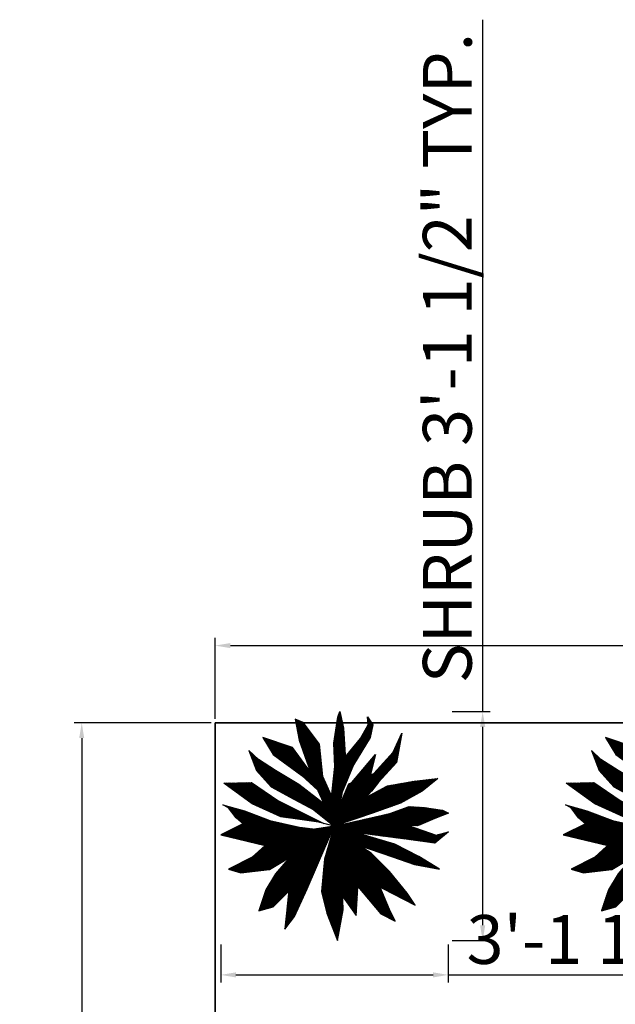
# Model space of a CAD drawing. Units: inches. Extents: x 1986 to 21484, y -1816 to 2016.
# Tile 48 of 85: x 3507 to 3604, y 1855 to 2016. Entities that reach past the tile are written whole.
import ezdxf

# ---------------------------------------------------------------- set-up
doc = ezdxf.new("R2010")
doc.units = ezdxf.units.IN
for name, color, linetype, lineweight in [('A-ANNO-DIMS', 2, 'Continuous', 18), ('C-PROP', 7, 'Continuous', 35), ('L-PLNT', 84, 'Continuous', 13), ('vfolhas', 114, 'Continuous', 5)]:
    doc.layers.add(name, color=color, linetype=linetype, lineweight=lineweight)
for name, color, linetype in [('vfolha', 72, 'Continuous'), ('vfolha2', 110, 'Continuous'), ('vfolhas2', 102, 'Continuous')]:
    doc.layers.add(name, color=color, linetype=linetype)
doc.styles.get("Standard").update_dxf_attribs({"font": 'arial.ttf'})
doc.dimstyles.new('ISO-25', dxfattribs={"dimtxt": 8, "dimasz": 2.5, "dimexe": 1.25, "dimexo": 0.625, "dimtad": 1, "dimdec": 1, "dimlunit": 3, "dimtxsty": 'Standard', "dimcen": 2.5, "dimadec": 0, "dimazin": 0, "dimtfac": 1, "dimtdec": 1, "dimtmove": 0, "dimatfit": 3, "dimfxl": 1, "dimarcsym": 0})
pattern_1 = [(45, (-2446.5133113, 50.986076), (-0.004419417382, 0.004419417382), [])]

# ---------------------------------------------------------------- blocks, each defined once
blk = doc.blocks.new('*D33')
at = {"layer": 'A-ANNO-DIMS', "color": 0, "lineweight": -2, "transparency": 16777216}
for p, q in [((3538.91, 1901.38), (3538.91, 1914.65)), ((3898.91, 1901.38), (3898.91, 1914.65)), ((3541.41, 1913.4), (3896.41, 1913.4))]:
    blk.add_line(p, q, dxfattribs=at)
at = {"layer": 'A-ANNO-DIMS', "color": 0, "transparency": 16777216}
for points in [[(3541.41, 1913.82), (3541.41, 1912.99), (3538.91, 1913.4)], [(3896.41, 1913.82), (3896.41, 1912.99), (3898.91, 1913.4)]]:
    blk.add_solid(points, dxfattribs=at)
at = {"layer": 'Defpoints', "color": 0, "transparency": 16777216}
for p in [(3898.91, 1913.4), (3538.91, 1900.75), (3898.91, 1900.75)]:
    blk.add_point(p, dxfattribs=at)
at = {"layer": 'A-ANNO-DIMS', "color": 0, "transparency": 16777216, "insert": (3718.91, 1918.12), "char_height": 8, "attachment_point": 5}
blk.add_mtext("30'", dxfattribs=at)
blk = doc.blocks.new('*D32')
at = {"layer": 'A-ANNO-DIMS', "color": 0, "lineweight": -2, "transparency": 16777216}
for p, q in [((3538.28, 1900.75), (3515.81, 1900.75)), ((3517.06, 1898.25), (3517.06, 1069.25)), ((3538.28, 1066.75), (3515.81, 1066.75))]:
    blk.add_line(p, q, dxfattribs=at)
at = {"layer": 'A-ANNO-DIMS', "color": 0, "transparency": 16777216}
for points in [[(3516.64, 1898.25), (3517.47, 1898.25), (3517.06, 1900.75)], [(3516.64, 1069.25), (3517.47, 1069.25), (3517.06, 1066.75)]]:
    blk.add_solid(points, dxfattribs=at)
at = {"layer": 'Defpoints', "color": 0, "transparency": 16777216}
for p in [(3538.91, 1900.75), (3517.06, 1066.75), (3538.91, 1066.75)]:
    blk.add_point(p, dxfattribs=at)
at = {"layer": 'A-ANNO-DIMS', "color": 0, "transparency": 16777216, "insert": (3512.35, 1483.75), "char_height": 8, "attachment_point": 5, "rotation": 90}
blk.add_mtext('69\'-6"', dxfattribs=at)
blk = doc.blocks.new('arbusto_PB_verde_grande')
at = {"layer": 'vfolha2'}
h = blk.add_hatch(dxfattribs=at)
h.set_pattern_fill('ANSI31', color=256, scale=0.05, style=0)
h.set_pattern_definition(pattern_1)
h.paths.add_polyline_path([(0.0294, 0.3565), (0.0003, 0.0905), (0.0263, -0.0393), (0.047, 0.0623), (0.0619, 0.0973), (0.0937, 0.2657), (0.0996, 0.4347), (0.0879, 0.6131), (0.0645, 0.7227), (0.0499, 0.6851), (0.0236, 0.5129)])
h.paths.add_polyline_path([(0.3011, 0.4379), (0.1423, 0.2487), (0.2669, 0.3002)])
h.paths.add_polyline_path([(0.38, 0.2282), (0.237, 0.1519), (0.1843, 0.0936), (0.1112, 0.0436), (0.0263, -0.0393), (0.2806, 0.0467), (0.3683, 0.078), (0.4676, 0.1124), (0.6107, 0.1938), (0.7159, 0.2782), (0.5581, 0.2595)])
h.paths.add_polyline_path([(0.561, -0.2944), (0.7275, -0.3257), (0.5902, -0.2412), (0.4296, -0.1598), (0.0263, -0.0393), (0.1492, -0.1411), (0.1884, -0.166), (0.415, -0.2444)])
h.paths.add_polyline_path([(-0.2743, -0.4478), (-0.3035, -0.7263), (-0.2392, -0.6417), (-0.1546, -0.4572), (0.0263, -0.0393), (-0.1633, -0.2538)])
h.paths.add_polyline_path([(-0.5196, -0.2474), (-0.6774, -0.3257), (-0.5956, -0.3507), (-0.4057, -0.3288), (-0.2101, -0.21), (0.0263, -0.0393), (-0.1487, -0.0659), (-0.3152, -0.091), (-0.4145, -0.1505)])
h.paths.add_polyline_path([(-0.5255, 0.2501), (-0.7095, 0.247), (-0.5196, 0.1093), (-0.3298, 0.0217), (-0.0757, -0.0128), (-0.0423, -0.0215), (-0.3502, 0.1312)])
h = blk.add_hatch(dxfattribs=at)
h.set_pattern_fill('ANSI31', color=256, scale=0.05, style=0)
h.set_pattern_definition(pattern_1)
h.paths.add_polyline_path([(-0.1896, 0.297), (-0.0855, 0.2019), (-0.1078, 0.2501), (-0.132, 0.3187), (-0.251, 0.4848), (-0.4495, 0.5505), (-0.3795, 0.4379)])
h.paths.add_polyline_path([(0.0791, -0.4071), (0.0821, -0.5063), (0.1726, -0.6355), (0.1843, -0.4415), (0.149, -0.2918), (0.0263, -0.0393), (0.0353, -0.2538)])
at = {"layer": 'vfolhas'}
h = blk.add_hatch(dxfattribs=at)
h.set_pattern_fill('ANSI31', color=256, scale=0.05, style=0)
h.set_pattern_definition(pattern_1)
h.paths.add_polyline_path([(-0.0728, 0.5067), (-0.1808, 0.6506), (-0.2334, 0.6725), (-0.2071, 0.5318), (-0.1078, 0.2501), (0.0263, -0.0393), (0.0003, 0.0905), (0.0082, 0.1624), (-0.0494, 0.2908)])
h.paths.add_polyline_path([(0.099, 0.4193), (0.0937, 0.2657), (0.0791, 0.1881), (0.1551, 0.369), (0.2661, 0.5505), (0.2836, 0.635), (0.2485, 0.6882), (0.2514, 0.635), (0.2018, 0.5443)])
h.paths.add_polyline_path([(0.1229, 0.2407), (0.047, 0.0623), (0.0263, -0.0393), (0.1112, 0.0436), (0.1843, 0.0936), (0.2748, 0.1938), (0.3215, 0.2532), (0.4413, 0.3847), (0.4763, 0.5787), (0.4179, 0.4535), (0.2894, 0.3095)])
h.paths.add_polyline_path([(0.5815, -0.0378), (0.7071, 0.0154), (0.7859, 0.0467), (0.748, 0.0655), (0.6282, 0.0842), (0.526, 0.0905), (0.3974, 0.0436), (0.0263, -0.0393), (0.2573, -0.0315), (0.4383, -0.0347)])
h.paths.add_polyline_path([(0.5202, -0.0365), (0.4383, -0.0347), (0.2573, -0.0315), (0.0263, -0.0393), (0.1796, -0.0852), (0.5377, -0.1317), (0.6954, -0.1536), (0.7859, -0.0785), (0.7041, -0.1004)])
h.paths.add_polyline_path([(0.2719, -0.2193), (0.1492, -0.1411), (0.0263, -0.0393), (0.1579, -0.3101), (0.2952, -0.4258), (0.4179, -0.4916), (0.564, -0.5667), (0.5114, -0.4853), (0.3946, -0.3414)])
h.paths.add_polyline_path([(-0.0582, -0.4759), (-0.0231, -0.6198), (0.047, -0.8013), (0.0849, -0.5979), (0.0791, -0.4071), (0.0353, -0.2538), (0.0263, -0.0393), (-0.0377, -0.26)])
h.paths.add_polyline_path([(-0.2422, 0.1405), (-0.1107, 0.0686), (0.0263, -0.0393), (-0.0423, 0.1087), (-0.2101, 0.2376), (-0.3649, 0.3314), (-0.4787, 0.4034), (-0.543, 0.4629), (-0.4904, 0.3314), (-0.3941, 0.2219)])
h = blk.add_hatch(dxfattribs=at)
h.set_pattern_fill('ANSI31', color=256, scale=0.05, style=0)
h.set_pattern_definition(pattern_1)
h.paths.add_polyline_path([(-0.5722, 0.0623), (-0.7153, 0.103), (-0.6774, 0.0811), (-0.6277, 0.0154), (-0.5635, -0.041), (-0.2646, -0.0834), (-0.1487, -0.0659), (-0.1015, -0.0588), (-0.2042, -0.0472), (-0.4028, -0.0034)])
h.paths.add_polyline_path([(-0.5635, -0.041), (-0.5828, -0.024), (-0.7299, -0.0973), (-0.4334, -0.1679), (-0.4145, -0.1505), (-0.3152, -0.091), (-0.2646, -0.0834)])
h.paths.add_polyline_path([(-0.2769, -0.4727), (-0.2743, -0.4478), (-0.1633, -0.2538), (0.0263, -0.0393), (-0.2101, -0.21), (-0.2672, -0.2447), (-0.3649, -0.357), (-0.4291, -0.4634), (-0.4759, -0.6043), (-0.3795, -0.576)])
h = blk.add_hatch(dxfattribs=at)
h.set_pattern_fill('ANSI31', color=256, scale=0.05, style=0)
h.set_pattern_definition(pattern_1)
h.paths.add_polyline_path([(0.3361, -0.623), (0.4325, -0.6731), (0.3946, -0.5948), (0.3303, -0.4446), (0.2952, -0.4258), (0.1579, -0.3101), (0.149, -0.2918), (0.1843, -0.4415)])
at = {"layer": 'vfolha'}
for p, q in [((0.0263, -0.0393), (-0.1487, -0.0659)), ((0.0263, -0.0393), (-0.0377, -0.26)), ((0.0353, -0.2538), (0.0263, -0.0393)), ((0.5202, -0.0365), (0.7041, -0.1004)), ((0.5377, -0.1317), (0.1796, -0.0852)), ((0.7859, -0.0785), (0.6954, -0.1536)), ((0.7041, -0.1004), (0.7859, -0.0785)), ((0.6954, -0.1536), (0.5377, -0.1317)), ((-0.2672, -0.2447), (-0.3649, -0.357)), ((-0.0377, -0.26), (-0.0582, -0.4759)), ((0.0791, -0.4071), (0.0353, -0.2538)), ((0.3946, -0.3414), (0.2719, -0.2193)), ((0.1579, -0.3101), (0.2952, -0.4258)), ((0.5114, -0.4853), (0.3946, -0.3414)), ((0.0849, -0.5979), (0.0791, -0.4071)), ((0.2952, -0.4258), (0.4179, -0.4916)), ((0.4179, -0.4916), (0.564, -0.5667)), ((0.564, -0.5667), (0.5114, -0.4853)), ((-0.0231, -0.6198), (0.047, -0.8013)), ((0.047, -0.8013), (0.0849, -0.5979))]:
    blk.add_line(p, q, dxfattribs=at)
at = {"layer": 'vfolha2'}
for p, q in [((0.0499, 0.6851), (0.0645, 0.7227)), ((0.0645, 0.7227), (0.0879, 0.6131)), ((0.0236, 0.5129), (0.0499, 0.6851)), ((0.0879, 0.6131), (0.0996, 0.4347)), ((-0.4495, 0.5505), (-0.3795, 0.4379)), ((-0.251, 0.4848), (-0.4495, 0.5505)), ((-0.132, 0.3187), (-0.251, 0.4848)), ((0.0294, 0.3565), (0.0236, 0.5129)), ((-0.3795, 0.4379), (-0.1896, 0.297)), ((0.0996, 0.4347), (0.0937, 0.2657)), ((0.1434, 0.2501), (0.3011, 0.4379)), ((0.3011, 0.4379), (0.2661, 0.297)), ((0.0003, 0.0905), (0.0294, 0.3565)), ((-0.1896, 0.297), (-0.0822, 0.1989)), ((0.5581, 0.2595), (0.7159, 0.2782)), ((0.7159, 0.2782), (0.6107, 0.1938)), ((-0.7095, 0.247), (-0.5255, 0.2501)), ((-0.5196, 0.1093), (-0.7095, 0.247)), ((-0.5255, 0.2501), (-0.3502, 0.1312)), ((0.237, 0.1519), (0.38, 0.2282)), ((0.38, 0.2282), (0.5581, 0.2595)), ((-0.3502, 0.1312), (-0.0423, -0.0215)), ((0.6107, 0.1938), (0.4676, 0.1124)), ((-0.3298, 0.0217), (-0.5196, 0.1093)), ((0.0263, -0.0393), (0.0003, 0.0905)), ((0.3683, 0.078), (0.2806, 0.0467)), ((-0.0757, -0.0128), (-0.3298, 0.0217)), ((0.2806, 0.0467), (0.0263, -0.0393)), ((-0.2101, -0.21), (0.0263, -0.0393)), ((0.0263, -0.0393), (-0.1633, -0.2538)), ((-0.1546, -0.4572), (0.0263, -0.0393)), ((0.4296, -0.1598), (0.0263, -0.0393)), ((0.0263, -0.0393), (0.1579, -0.3101)), ((-0.3152, -0.091), (-0.4145, -0.1505)), ((-0.1487, -0.0659), (-0.3152, -0.091)), ((-0.4145, -0.1505), (-0.5196, -0.2474)), ((0.1884, -0.166), (0.415, -0.2444)), ((0.5902, -0.2412), (0.4296, -0.1598)), ((-0.5196, -0.2474), (-0.6774, -0.3257)), ((-0.4057, -0.3288), (-0.2101, -0.21)), ((-0.1633, -0.2538), (-0.2743, -0.4478)), ((0.415, -0.2444), (0.561, -0.2944)), ((0.7275, -0.3257), (0.5902, -0.2412)), ((-0.6774, -0.3257), (-0.5956, -0.3507)), ((0.1843, -0.4415), (0.149, -0.2918)), ((0.561, -0.2944), (0.7275, -0.3257)), ((-0.5956, -0.3507), (-0.4057, -0.3288)), ((-0.2743, -0.4478), (-0.3035, -0.7263)), ((0.1726, -0.6355), (0.1843, -0.4415)), ((0.0821, -0.5063), (0.1726, -0.6355)), ((-0.3035, -0.7263), (-0.2392, -0.6417))]:
    blk.add_line(p, q, dxfattribs=at)
at = {"layer": 'vfolhas2'}
for p, q in [((-0.2334, 0.6725), (-0.2071, 0.5318)), ((-0.1808, 0.6506), (-0.2334, 0.6725)), ((0.2514, 0.635), (0.2485, 0.6882)), ((0.2485, 0.6882), (0.2836, 0.635)), ((-0.0728, 0.5067), (-0.1808, 0.6506)), ((0.2018, 0.5443), (0.2514, 0.635)), ((0.2836, 0.635), (0.2661, 0.5505)), ((-0.2071, 0.5318), (-0.1078, 0.2501)), ((0.099, 0.4193), (0.2018, 0.5443)), ((0.2661, 0.5505), (0.1551, 0.369)), ((0.4179, 0.4535), (0.4763, 0.5787)), ((0.4763, 0.5787), (0.4413, 0.3847)), ((-0.543, 0.4629), (-0.4904, 0.3314)), ((-0.4787, 0.4034), (-0.543, 0.4629)), ((-0.0494, 0.2908), (-0.0728, 0.5067)), ((-0.3649, 0.3314), (-0.4787, 0.4034)), ((0.2894, 0.3095), (0.4179, 0.4535)), ((-0.4904, 0.3314), (-0.3941, 0.2219)), ((-0.2101, 0.2376), (-0.3649, 0.3314)), ((0.1551, 0.369), (0.078, 0.1855)), ((0.4413, 0.3847), (0.3215, 0.2532)), ((0.0082, 0.1624), (-0.0494, 0.2908)), ((0.0937, 0.2657), (0.0619, 0.0973)), ((0.1229, 0.2407), (0.2894, 0.3095)), ((-0.3941, 0.2219), (-0.2422, 0.1405)), ((-0.0423, 0.1087), (-0.2101, 0.2376)), ((-0.1078, 0.2501), (0.0263, -0.0393)), ((0.047, 0.0623), (0.1229, 0.2407)), ((0.3215, 0.2532), (0.2748, 0.1938)), ((-0.2422, 0.1405), (-0.1107, 0.0686)), ((0.2748, 0.1938), (0.1843, 0.0936)), ((-0.6774, 0.0811), (-0.7153, 0.103)), ((-0.7153, 0.103), (-0.5722, 0.0623)), ((-0.6277, 0.0154), (-0.6774, 0.0811)), ((-0.1107, 0.0686), (0.0263, -0.0393)), ((0.1843, 0.0936), (0.1112, 0.0436)), ((0.4676, 0.1124), (0.3683, 0.078)), ((0.3974, 0.0436), (0.526, 0.0905)), ((0.526, 0.0905), (0.6282, 0.0842)), ((0.6282, 0.0842), (0.748, 0.0655)), ((-0.5635, -0.041), (-0.6277, 0.0154)), ((-0.5722, 0.0623), (-0.4028, -0.0034)), ((0.0263, -0.0393), (0.047, 0.0623)), ((0.0263, -0.0393), (0.3974, 0.0436)), ((0.1112, 0.0436), (0.0263, -0.0393)), ((0.7071, 0.0154), (0.5815, -0.0378)), ((0.7859, 0.0467), (0.7071, 0.0154)), ((0.748, 0.0655), (0.7859, 0.0467)), ((-0.5828, -0.024), (-0.7299, -0.0973)), ((-0.2646, -0.0834), (-0.5635, -0.041)), ((-0.4028, -0.0034), (-0.2042, -0.0472)), ((-0.2042, -0.0472), (-0.0983, -0.0591)), ((0.0263, -0.0393), (-0.0757, -0.0128)), ((0.2573, -0.0315), (0.0263, -0.0393)), ((0.1492, -0.1411), (0.0263, -0.0393)), ((0.4383, -0.0347), (0.2573, -0.0315)), ((0.5815, -0.0378), (0.4383, -0.0347)), ((-0.7299, -0.0973), (-0.4334, -0.1679)), ((0.2719, -0.2193), (0.1492, -0.1411)), ((-0.3649, -0.357), (-0.4291, -0.4634)), ((-0.2392, -0.6417), (-0.1546, -0.4572)), ((0.1843, -0.4415), (0.3361, -0.623)), ((0.3946, -0.5948), (0.329, -0.4417)), ((-0.4291, -0.4634), (-0.4759, -0.6043)), ((-0.3795, -0.576), (-0.2769, -0.4727)), ((-0.0582, -0.4759), (-0.0231, -0.6198)), ((-0.4759, -0.6043), (-0.3795, -0.576)), ((0.3361, -0.623), (0.4325, -0.6731)), ((0.4325, -0.6731), (0.3946, -0.5948))]:
    blk.add_line(p, q, dxfattribs=at)
blk = doc.blocks.new('*D95')
at = {"layer": 'A-ANNO-DIMS', "color": 0, "lineweight": -2, "transparency": 16777216}
for p, q in [((3582.74, 1902.59), (3582.74, 2015.93)), ((3577.74, 1902.59), (3583.99, 1902.59)), ((3582.74, 1867.59), (3582.74, 1900.09)), ((3577.74, 1865.09), (3583.99, 1865.09))]:
    blk.add_line(p, q, dxfattribs=at)
at = {"layer": 'A-ANNO-DIMS', "color": 0, "transparency": 16777216}
for points in [[(3582.32, 1900.09), (3583.16, 1900.09), (3582.74, 1902.59)], [(3582.32, 1867.59), (3583.16, 1867.59), (3582.74, 1865.09)]]:
    blk.add_solid(points, dxfattribs=at)
at = {"layer": 'Defpoints', "color": 0, "transparency": 16777216}
for p in [(3577.11, 1902.59), (3582.74, 1902.59), (3577.11, 1865.09)]:
    blk.add_point(p, dxfattribs=at)
at = {"layer": 'A-ANNO-DIMS', "color": 0, "transparency": 16777216, "insert": (3577.98, 1960.51), "char_height": 8, "attachment_point": 5, "rotation": 90}
blk.add_mtext('SHRUB 3\'-1 1/2" TYP.', dxfattribs=at)
blk = doc.blocks.new('*D96')
at = {"layer": 'A-ANNO-DIMS', "color": 0, "lineweight": -2, "transparency": 16777216}
for p, q in [((3539.82, 1864.46), (3539.82, 1858.21)), ((3577.11, 1864.46), (3577.11, 1858.21)), ((3542.32, 1859.46), (3574.61, 1859.46)), ((3577.11, 1859.46), (3648.26, 1859.46))]:
    blk.add_line(p, q, dxfattribs=at)
at = {"layer": 'A-ANNO-DIMS', "color": 0, "transparency": 16777216}
for points in [[(3542.32, 1859.88), (3542.32, 1859.05), (3539.82, 1859.46)], [(3574.61, 1859.88), (3574.61, 1859.05), (3577.11, 1859.46)]]:
    blk.add_solid(points, dxfattribs=at)
at = {"layer": 'Defpoints', "color": 0, "transparency": 16777216}
for p in [(3539.82, 1865.09), (3577.11, 1865.09), (3577.11, 1859.46)]:
    blk.add_point(p, dxfattribs=at)
at = {"layer": 'A-ANNO-DIMS', "color": 0, "transparency": 16777216, "insert": (3613.94, 1864.23), "char_height": 8, "attachment_point": 5}
blk.add_mtext('3\'-1 1/2" TYP.', dxfattribs=at)

msp = doc.modelspace()

# ---------------------------------------------------------------- linework, layer by layer
at = {"layer": 'C-PROP'}
msp.add_lwpolyline([(3538.91, 1900.75), (3898.91, 1900.75), (3898.91, 1066.75), (3538.91, 1066.75)], close=True, dxfattribs=at)

# ---------------------------------------------------------------- block references
at = {"layer": 'L-PLNT', "xscale": 24.60366729364114, "yscale": 24.60366729364114, "zscale": 24.60366729364114}
for p in [(3557.78, 1884.81), (3613.9, 1884.81)]:
    msp.add_blockref('arbusto_PB_verde_grande', p, dxfattribs=at)

# ---------------------------------------------------------------- dimensions: what is measured, and where the dimension line sits
at = {"layer": 'A-ANNO-DIMS'}
dim = msp.add_linear_dim(base=(3582.74, 1902.59), p1=(3577.11, 1865.09), p2=(3577.11, 1902.59), angle=90, text='SHRUB <> TYP.', dimstyle='ISO-25', override={"dimdec": 1, "dimrnd": 0, "dimzin": 1, "dimlunit": 4, "dimfrac": 2}, dxfattribs=at)
dim.commit()
dim.dimension.update_dxf_attribs({"geometry": '*D95', "text_midpoint": (3577.98, 1960.51)})
dim = msp.add_linear_dim(base=(3898.91, 1913.4), p1=(3538.91, 1900.75), p2=(3898.91, 1900.75), dimstyle='ISO-25', override={"dimclrd": 0, "dimclre": 0, "dimclrt": 0}, dxfattribs=at)
dim.commit()
dim.dimension.update_dxf_attribs({"geometry": '*D33', "text_midpoint": (3718.91, 1918.12)})
dim = msp.add_linear_dim(base=(3517.06, 1066.75), p1=(3538.91, 1900.75), p2=(3538.91, 1066.75), angle=90, dimstyle='ISO-25', override={"dimclrd": 0, "dimclre": 0, "dimclrt": 0}, dxfattribs=at)
dim.commit()
dim.dimension.update_dxf_attribs({"geometry": '*D32', "text_midpoint": (3512.35, 1483.75)})
dim = msp.add_linear_dim(base=(3577.11, 1859.46), p1=(3539.82, 1865.09), p2=(3577.11, 1865.09), text='<> TYP.', dimstyle='ISO-25', override={"dimdec": 1, "dimrnd": 0, "dimzin": 1, "dimlunit": 4, "dimfrac": 2}, dxfattribs=at)
dim.commit()
dim.dimension.update_dxf_attribs({"geometry": '*D96', "text_midpoint": (3613.94, 1864.23)})

doc.saveas('drawing.dxf')
